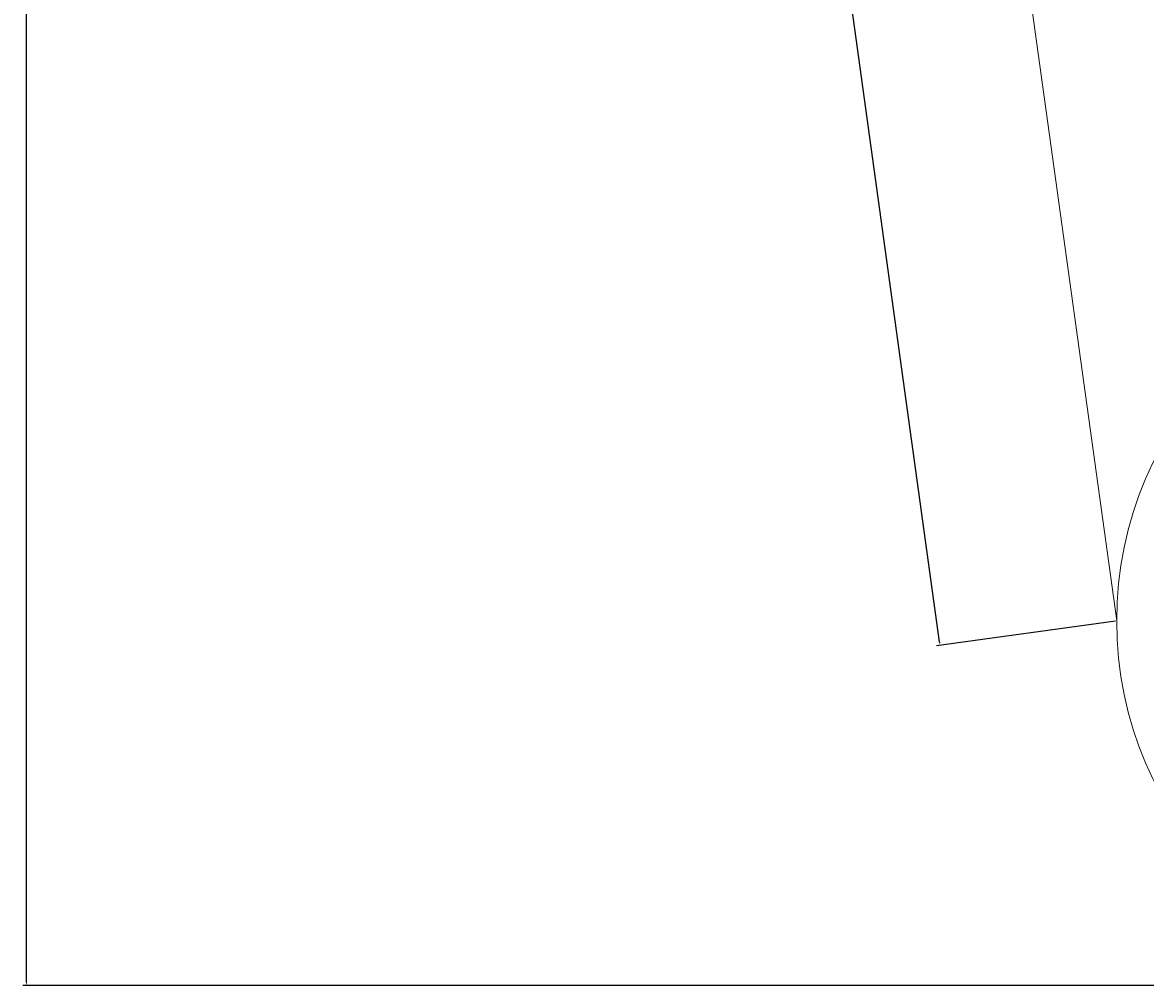
# Model space of a CAD drawing. Units: millimetres. Extents: x -9 to 135, y -119 to 27.
# Tile 1 of 12: x -9 to 46, y -110 to -63. Entities that reach past the tile are written whole.
import ezdxf

# ---------------------------------------------------------------- set-up
doc = ezdxf.new("R2010")
doc.units = ezdxf.units.MM
doc.layers.add('M-CONS', color=8, linetype='Continuous', lineweight=18)
doc.layers.add('M-DIMS', color=2, linetype='Continuous', lineweight=18)
doc.styles.get("Standard").update_dxf_attribs({"font": 'arial.ttf'})
doc.dimstyles.get("Standard").update_dxf_attribs({"dimtxt": 0.18, "dimasz": 0.18, "dimexe": 0.18, "dimexo": 0.0625, "dimgap": 0.09, "dimtad": 0, "dimtih": 1, "dimtoh": 1, "dimdec": 4, "dimzin": 0, "dimdsep": 46, "dimtxsty": 'Standard', "dimcen": 0.09, "dimadec": 0, "dimazin": 0, "dimtfac": 1, "dimtdec": 4, "dimtofl": 0, "dimtmove": 0, "dimatfit": 3, "dimfxl": 1, "dimtolj": 1, "dimtzin": 0, "dimarcsym": 0})

# ---------------------------------------------------------------- blocks, each defined once
blk = doc.blocks.new('*D3')
at = {"layer": 'Defpoints', "color": 0, "transparency": 16777216}
for p in [(0, 17.733), (-8.8, -110.267), (63, -110.267)]:
    blk.add_point(p, dxfattribs=at)
at = {"layer": 'M-DIMS', "color": 0, "lineweight": -2, "transparency": 16777216}
for p, q in [((-0.062, 17.733), (-8.98, 17.733)), ((-8.8, 17.553), (-8.8, -46.085)), ((-8.8, -110.087), (-8.8, -46.449)), ((62.938, -110.267), (-8.98, -110.267))]:
    blk.add_line(p, q, dxfattribs=at)
at = {"layer": 'M-DIMS', "color": 0, "transparency": 16777216}
for points in [[(-8.83, 17.553), (-8.77, 17.553), (-8.8, 17.733)], [(-8.83, -110.087), (-8.77, -110.087), (-8.8, -110.267)]]:
    blk.add_solid(points, dxfattribs=at)
at = {"layer": 'M-DIMS', "color": 0, "transparency": 16777216, "insert": (-8.8, -46.267), "char_height": 0.18, "attachment_point": 5}
blk.add_mtext('\\A1;128', dxfattribs=at)
blk = doc.blocks.new('*D14')
at = {"layer": 'Defpoints', "color": 0, "transparency": 16777216}
for p in [(32, 1.733), (23.283, 0.528), (45, -92.267)]:
    blk.add_point(p, dxfattribs=at)
at = {"layer": 'M-DIMS', "color": 0, "lineweight": -2, "transparency": 16777216}
for p, q in [((31.938, 1.725), (23.105, 0.503)), ((23.308, 0.349), (29.758, -46.29)), ((36.258, -93.294), (29.808, -46.654)), ((44.938, -92.275), (36.105, -93.497))]:
    blk.add_line(p, q, dxfattribs=at)
at = {"layer": 'M-DIMS', "color": 0, "transparency": 16777216}
for points in [[(23.337, 0.353), (23.278, 0.345), (23.283, 0.528)], [(36.288, -93.29), (36.229, -93.298), (36.283, -93.472)]]:
    blk.add_solid(points, dxfattribs=at)
at = {"layer": 'M-DIMS', "color": 0, "transparency": 16777216, "insert": (29.783, -46.472), "char_height": 0.18, "attachment_point": 5}
blk.add_mtext('\\A1;94.9', dxfattribs=at)

msp = doc.modelspace()

# ---------------------------------------------------------------- linework, layer by layer
at = {"layer": 'M-CONS'}
msp.add_line((32, 1.733, 115.129), (45, -92.267, 115.129), dxfattribs=at)
msp.add_circle((63, -92.267, 115.129), 18, dxfattribs=at)

# ---------------------------------------------------------------- dimensions: what is measured, and where the dimension line sits
at = {"layer": 'M-DIMS'}
for base, p1, p2, angle, override, picture, middle in [((-8.8, -110.267), (0, 17.733), (63, -110.267), 90, {"dimdec": 0, "dimlfac": 1, "dimrnd": 0, "dimzin": 0, "dimdsep": 46, "dimlunit": 2}, '*D3', (-8.8, -46.267)), ((23.283, 0.528), (45, -92.267), (32, 1.733), 97.8739, {"dimdec": 1, "dimlfac": 1, "dimrnd": 0, "dimzin": 0, "dimdsep": 46, "dimlunit": 2}, '*D14', (29.783, -46.472))]:
    dim = msp.add_linear_dim(base=base, p1=p1, p2=p2, angle=angle, dimstyle='Standard', override=override, dxfattribs=at)
    dim.commit()
    dim.dimension.update_dxf_attribs({"geometry": picture, "text_midpoint": middle})

doc.saveas('drawing.dxf')
